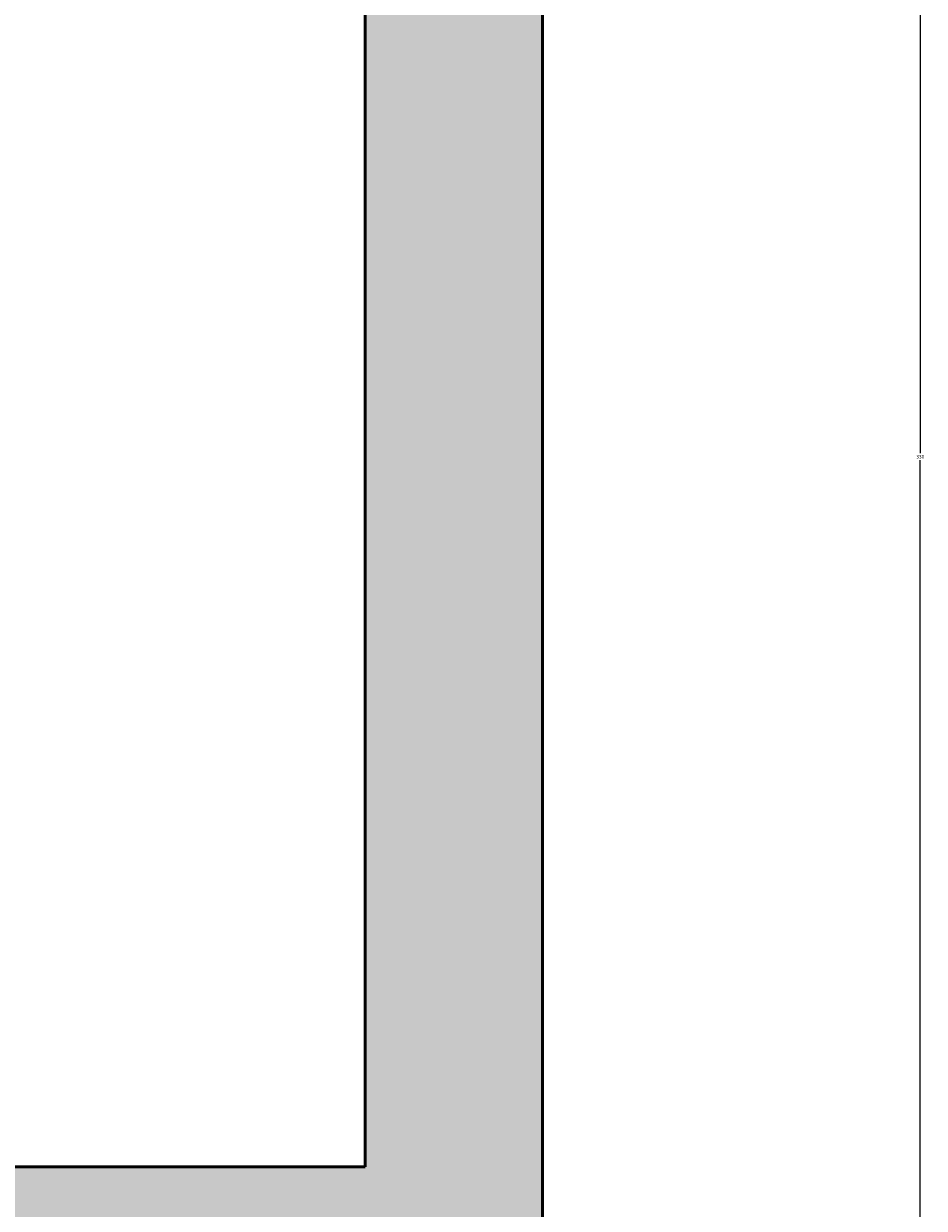
# Model space of a CAD drawing. Units: inches. Extents: x 2307 to 2544, y 2171 to 2540.
# Tile 33 of 52: x 2498 to 2544, y 2317 to 2377. Entities that reach past the tile are written whole.
import ezdxf

# ---------------------------------------------------------------- set-up
doc = ezdxf.new("R2010")
doc.units = ezdxf.units.IN
doc.layers.add('A-ANNO-DIMS', color=2, linetype='Continuous', lineweight=18)
doc.layers.add('A-WALL', color=7, linetype='Continuous', lineweight=50)
doc.layers.add('A-WALL-PATT', color=18, linetype='Continuous', lineweight=13, true_color=0x000000)
doc.styles.get("Standard").update_dxf_attribs({"font": 'arial.ttf'})
doc.dimstyles.get("Standard").update_dxf_attribs({"dimtxt": 0.18, "dimasz": 0.18, "dimexe": 0.18, "dimexo": 0.0625, "dimgap": 0.09, "dimtad": 0, "dimtih": 1, "dimtoh": 1, "dimdec": 4, "dimzin": 0, "dimdsep": 46, "dimtxsty": 'Standard', "dimcen": 0.09, "dimadec": 0, "dimazin": 0, "dimtfac": 1, "dimtdec": 4, "dimtofl": 0, "dimtmove": 0, "dimatfit": 3, "dimfxl": 1, "dimtolj": 1, "dimtzin": 0, "dimarcsym": 0})

# ---------------------------------------------------------------- blocks, each defined once
blk = doc.blocks.new('*D37')
at = {"layer": 'A-ANNO-DIMS', "color": 0, "lineweight": -2, "transparency": 16777216}
for p, q in [((2524.758, 2520.51), (2544.026, 2520.51)), ((2543.846, 2520.33), (2543.846, 2355.692)), ((2543.846, 2190.69), (2543.846, 2355.328)), ((2524.758, 2190.51), (2544.026, 2190.51))]:
    blk.add_line(p, q, dxfattribs=at)
at = {"layer": 'A-ANNO-DIMS', "color": 0, "transparency": 16777216}
for points in [[(2543.816, 2520.33), (2543.876, 2520.33), (2543.846, 2520.51)], [(2543.816, 2190.69), (2543.876, 2190.69), (2543.846, 2190.51)]]:
    blk.add_solid(points, dxfattribs=at)
at = {"layer": 'Defpoints', "color": 0, "transparency": 16777216}
for p in [(2524.696, 2520.51), (2543.846, 2520.51), (2524.696, 2190.51)]:
    blk.add_point(p, dxfattribs=at)
at = {"layer": 'A-ANNO-DIMS', "color": 0, "transparency": 16777216, "insert": (2543.846, 2355.51), "char_height": 0.18, "attachment_point": 5}
blk.add_mtext('\\A1;330', dxfattribs=at)

msp = doc.modelspace()

# ---------------------------------------------------------------- hatches: boundary and pattern name
at = {"layer": 'A-WALL-PATT'}
h = msp.add_hatch(color=256, dxfattribs=at)
h.dxf.hatch_style = 1
h.paths.add_polyline_path([(2433.6935, 2199.5096), (2415.6423, 2199.5096), (2415.6423, 2190.5096), (2433.7832, 2190.5096)], flags=17)
h.paths.add_polyline_path([(2367.6423, 2199.5096), (2335.6958, 2199.5096), (2335.6958, 2307.3983), (2326.6958, 2307.3983), (2326.6958, 2190.5096), (2367.6423, 2190.5096)])
h.paths.add_polyline_path([(2524.6958, 2520.5096), (2496.7832, 2520.5096), (2496.7832, 2515.5149), (2472.7832, 2515.5149), (2472.7832, 2520.5096), (2415.4028, 2520.5096), (2415.4028, 2511.5096), (2451.6958, 2511.5096), (2451.6958, 2439.5096), (2451.6958, 2391.5096), (2445.6958, 2391.5096), (2445.6958, 2387.5096), (2455.6958, 2387.5096), (2455.6958, 2435.5096), (2461.6958, 2435.5096), (2461.6958, 2439.5096), (2455.6958, 2439.5096), (2455.6958, 2511.5096), (2515.6958, 2511.5096), (2515.6958, 2439.5096), (2491.6958, 2439.5096), (2491.6958, 2435.5096), (2515.6958, 2435.5096), (2515.6958, 2319.5096), (2451.6958, 2319.5096), (2451.6958, 2281.5096), (2481.6958, 2281.5096), (2481.6958, 2225.5096), (2485.6958, 2225.5096), (2485.6958, 2285.5096), (2455.6958, 2285.5096), (2455.6958, 2315.5096), (2515.6958, 2315.5096), (2515.6958, 2199.5096), (2469.6952, 2199.5096), (2469.785, 2190.5096), (2524.6958, 2190.5096)])

# ---------------------------------------------------------------- linework, layer by layer
at = {"layer": 'A-WALL'}
for p, q in [((2515.6958, 2435.5096), (2515.6958, 2319.5096)), ((2515.6958, 2319.5096), (2451.6958, 2319.5096))]:
    msp.add_line(p, q, dxfattribs=at)
msp.add_lwpolyline([(2433.7832, 2190.5096), (2326.6958, 2190.5096), (2326.6958, 2520.5096), (2524.6958, 2520.5096), (2524.6958, 2190.5096), (2469.785, 2190.5096)], dxfattribs=at)

# ---------------------------------------------------------------- dimensions: what is measured, and where the dimension line sits
at = {"layer": 'A-ANNO-DIMS'}
dim = msp.add_linear_dim(base=(2543.8458, 2520.5096), p1=(2524.6958, 2190.5096), p2=(2524.6958, 2520.5096), angle=90, dimstyle='Standard', override={"dimdec": 0, "dimlfac": 1, "dimrnd": 0, "dimzin": 0, "dimdsep": 46, "dimlunit": 2}, dxfattribs=at)
dim.commit()
dim.dimension.update_dxf_attribs({"geometry": '*D37', "text_midpoint": (2543.8458, 2355.5096)})

doc.saveas('drawing.dxf')
